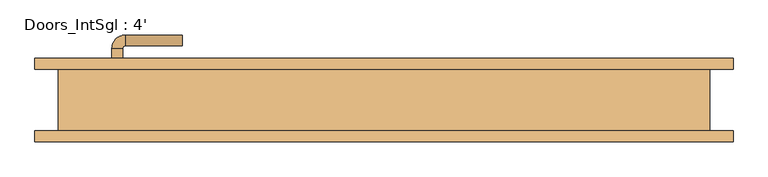
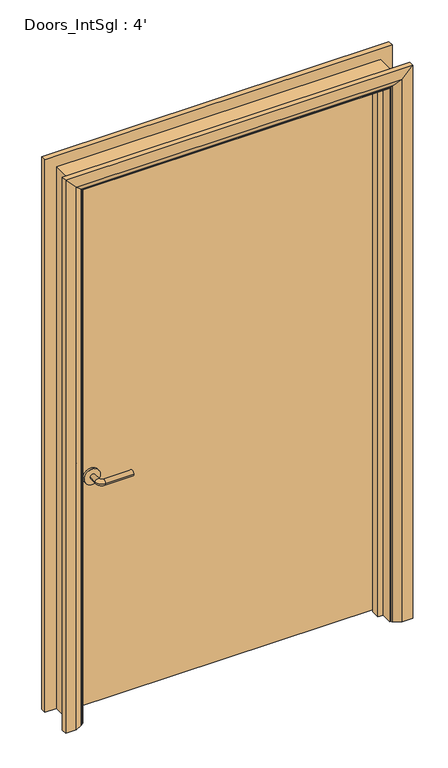
"""IFC4 building model written with IfcOpenShell, lengths in millimetres: door geometry, Doors_IntSgl : 4'."""

from ifc_helpers import new_model, si_unit, point, frame, frame_2d, origin, place, context, project, spatial, polyline, circle_curve, ellipse_curve, trimmed, segment, composite_curve, outline, extrude, faceted_brep, source, transform, mapped, element, save
from ifc_brep_helpers import plane_surface, cylinder_surface, revolved_surface, advanced_brep


def doors_intsgl_4_134d4d27(model_context):
    return source(origin(), model_context, "Body", "SolidModel", [
        advanced_brep(
        [(-502.6, 11.15, 900.0), (-482.6, 11.15, 900.0), (-482.6, -18.85, 900.0), (-502.6, -18.85, 900.0), (-477.6, -23.85, 900.0), (-477.6, -43.85, 900.0), (-372.6, -43.85, 900.0), (-372.6, -23.85, 900.0)],
        [
            (0, 1, circle_curve(frame((-492.6, 11.15, 900.0), z_axis=(0.0, 1.0, 0.0), x_axis=(1.0, 0.0, 0.0)), 10.0)),
            (1, 0, circle_curve(frame((-492.6, 11.15, 900.0), z_axis=(0.0, 1.0, 0.0), x_axis=(1.0, 0.0, 0.0)), 10.0)),
            (1, 2),
            (2, 3, circle_curve(frame((-492.6, -18.85, 900.0), z_axis=(0.0, 1.0, 0.0), x_axis=(1.0, 0.0, 0.0)), 10.0)),
            (3, 0),
            (3, 2, circle_curve(frame((-492.6, -18.85, 900.0), z_axis=(0.0, 1.0, 0.0), x_axis=(1.0, 0.0, 0.0)), 10.0)),
            (4, 5, circle_curve(frame((-477.6, -33.85, 900.0), z_axis=(-1.0, 0.0, 0.0), x_axis=(0.0, 1.0, 0.0)), 10.0)),
            (5, 3, circle_curve(frame((-477.6, -18.85, 900.0), z_axis=(0.0, 0.0, -1.0), x_axis=(-1.0, 0.0, 0.0)), 25.0)),
            (2, 4, circle_curve(frame((-477.6, -18.85, 900.0), z_axis=(0.0, 0.0, 1.0), x_axis=(-1.0, 0.0, 0.0)), 5.0)),
            (5, 4, circle_curve(frame((-477.6, -33.85, 900.0), z_axis=(-1.0, 0.0, 0.0), x_axis=(0.0, 1.0, 0.0)), 10.0)),
            (6, 7, circle_curve(frame((-372.6, -33.85, 900.0), z_axis=(1.0, 0.0, 0.0), x_axis=(0.0, 1.0, 0.0)), 10.0)),
            (7, 6, circle_curve(frame((-372.6, -33.85, 900.0), z_axis=(1.0, 0.0, 0.0), x_axis=(0.0, 1.0, 0.0)), 10.0)),
            (4, 7),
            (6, 5),
        ],
        [
            plane_surface(frame((-492.6, 11.15, 900.0), z_axis=(0.0, 1.0, 0.0), x_axis=(0.0, 0.0, 1.0))),
            cylinder_surface(frame((-492.6, 11.15, 900.0), z_axis=(0.0, 1.0, 0.0), x_axis=(1.0, 0.0, 0.0)), 10.0),
            revolved_surface(trimmed(ellipse_curve(frame((-492.6, -18.85, 900.0), z_axis=(0.0, -1.0, 0.0), x_axis=(1.0, 0.0, 0.0)), 10.0, 10.0), [point((-502.6, -18.85, 900.0))], [point((-482.6, -18.85, 900.0))], True, "CARTESIAN"), (-477.6, -18.85, 900.0), (0.0, 0.0, -1.0)),
            revolved_surface(trimmed(ellipse_curve(frame((-492.6, -18.85, 900.0), z_axis=(0.0, -1.0, 0.0), x_axis=(1.0, 0.0, 0.0)), 10.0, 10.0), [point((-482.6, -18.85, 900.0))], [point((-502.6, -18.85, 900.0))], True, "CARTESIAN"), (-477.6, -18.85, 900.0), (0.0, 0.0, -1.0)),
            plane_surface(frame((-372.6, -33.85, 900.0), z_axis=(1.0, 0.0, 0.0), x_axis=(0.0, 0.0, 1.0))),
            cylinder_surface(frame((-477.6, -33.85, 900.0), z_axis=(-1.0, 0.0, 0.0), x_axis=(0.0, 1.0, 0.0)), 10.0),
        ],
        [
            (0, [[1, 2]]),
            (1, [[3, 4, 5, -2]]),
            (1, [[-5, 6, -3, -1]]),
            (2, [[7, 8, -4, 9]]),
            (3, [[10, -9, -6, -8]]),
            (4, [[11, 12]]),
            (5, [[13, -11, 14, -7]]),
            (5, [[-14, -12, -13, -10]]),
        ],
    ),
        extrude(outline(composite_curve([segment(trimmed(circle_curve(frame_2d((900.0, -495.1)), 30.0), [point((900.0, -525.1))], [point((900.0, -465.1))], False, "CARTESIAN"), True, "CONTINUOUS"), segment(trimmed(circle_curve(frame_2d((900.0, -495.1)), 30.0), [point((900.0, -465.1))], [point((900.0, -525.1))], False, "CARTESIAN"), True, "CONTINUOUS")], self_intersect=False)), frame((0.0, 11.15, 0.0), z_axis=(0.0, 1.0, 0.0), x_axis=(0.0, 0.0, 1.0)), (0.0, 0.0, 1.0), 8.0),
        advanced_brep(
        [(-502.6, 65.15, 900.0), (-482.6, 65.15, 900.0), (-502.6, 95.15, 900.0), (-482.6, 95.15, 900.0), (-477.6, 100.15, 900.0), (-477.6, 120.15, 900.0), (-372.6, 120.15, 900.0), (-372.6, 100.15, 900.0)],
        [
            (0, 1, circle_curve(frame((-492.6, 65.15, 900.0), z_axis=(0.0, -1.0, 0.0), x_axis=(1.0, 0.0, 0.0)), 10.0)),
            (1, 0, circle_curve(frame((-492.6, 65.15, 900.0), z_axis=(0.0, -1.0, 0.0), x_axis=(1.0, 0.0, 0.0)), 10.0)),
            (0, 2),
            (2, 3, circle_curve(frame((-492.6, 95.15, 900.0), z_axis=(0.0, -1.0, 0.0), x_axis=(1.0, 0.0, 0.0)), 10.0)),
            (3, 1),
            (3, 2, circle_curve(frame((-492.6, 95.15, 900.0), z_axis=(0.0, -1.0, 0.0), x_axis=(1.0, 0.0, 0.0)), 10.0)),
            (4, 3, circle_curve(frame((-477.6, 95.15, 900.0), z_axis=(0.0, 0.0, 1.0), x_axis=(-1.0, 0.0, 0.0)), 5.0)),
            (2, 5, circle_curve(frame((-477.6, 95.15, 900.0), z_axis=(0.0, 0.0, -1.0), x_axis=(-1.0, 0.0, 0.0)), 25.0)),
            (5, 4, circle_curve(frame((-477.6, 110.15, 900.0), z_axis=(-1.0, 0.0, 0.0), x_axis=(0.0, -1.0, 0.0)), 10.0)),
            (4, 5, circle_curve(frame((-477.6, 110.15, 900.0), z_axis=(-1.0, 0.0, 0.0), x_axis=(0.0, -1.0, 0.0)), 10.0)),
            (6, 7, circle_curve(frame((-372.6, 110.15, 900.0), z_axis=(1.0, 0.0, 0.0), x_axis=(0.0, -1.0, 0.0)), 10.0)),
            (7, 6, circle_curve(frame((-372.6, 110.15, 900.0), z_axis=(1.0, 0.0, 0.0), x_axis=(0.0, -1.0, 0.0)), 10.0)),
            (5, 6),
            (7, 4),
        ],
        [
            plane_surface(frame((-492.6, 65.15, 900.0), z_axis=(0.0, -1.0, 0.0), x_axis=(0.0, 0.0, 1.0))),
            cylinder_surface(frame((-492.6, 65.15, 900.0), z_axis=(0.0, -1.0, 0.0), x_axis=(1.0, 0.0, 0.0)), 10.0),
            revolved_surface(trimmed(ellipse_curve(frame((-492.6, 95.15, 900.0), z_axis=(0.0, -1.0, 0.0), x_axis=(1.0, 0.0, 0.0)), 10.0, 10.0), [point((-502.6, 95.15, 900.0))], [point((-482.6, 95.15, 900.0))], True, "CARTESIAN"), (-477.6, 95.15, 900.0), (0.0, 0.0, -1.0)),
            revolved_surface(trimmed(ellipse_curve(frame((-492.6, 95.15, 900.0), z_axis=(0.0, -1.0, 0.0), x_axis=(1.0, 0.0, 0.0)), 10.0, 10.0), [point((-482.6, 95.15, 900.0))], [point((-502.6, 95.15, 900.0))], True, "CARTESIAN"), (-477.6, 95.15, 900.0), (0.0, 0.0, -1.0)),
            plane_surface(frame((-372.6, 110.15, 900.0), z_axis=(1.0, 0.0, 0.0), x_axis=(0.0, 0.0, 1.0))),
            cylinder_surface(frame((-477.6, 110.15, 900.0), z_axis=(-1.0, 0.0, 0.0), x_axis=(0.0, -1.0, 0.0)), 10.0),
        ],
        [
            (0, [[1, 2]]),
            (1, [[-1, 3, 4, 5]]),
            (1, [[-2, -5, 6, -3]]),
            (2, [[7, -4, 8, 9]]),
            (3, [[-8, -6, -7, 10]]),
            (4, [[11, 12]]),
            (5, [[-9, 13, -12, 14]]),
            (5, [[-10, -14, -11, -13]]),
        ],
    ),
        extrude(outline(composite_curve([segment(trimmed(circle_curve(frame_2d((900.0, -495.1)), 30.0), [point((900.0, -525.1))], [point((900.0, -465.1))], False, "CARTESIAN"), True, "CONTINUOUS"), segment(trimmed(circle_curve(frame_2d((900.0, -495.1)), 30.0), [point((900.0, -465.1))], [point((900.0, -525.1))], False, "CARTESIAN"), True, "CONTINUOUS")], self_intersect=False)), frame((0.0, 57.15, 0.0), z_axis=(0.0, 1.0, 0.0), x_axis=(0.0, 0.0, 1.0)), (0.0, 0.0, 1.0), 8.0),
        extrude(outline(polyline([(567.6, 19.15), (-567.6, 19.15), (-567.6, 57.15), (567.6, 57.15), (567.6, 19.15)])), frame((0.0, 0.0, 8.0), z_axis=(0.0, 0.0, 1.0), x_axis=(1.0, 0.0, 0.0)), (0.0, 0.0, 1.0), 2083.6),
        advanced_brep(
        [(644.6, 77.15, 0.0), (644.6, 57.15, 0.0), (574.6, 57.15, 0.0), (578.6, 63.15, 0.0), (604.6, 77.15, 0.0), (644.6, 77.15, 2168.6), (644.6, 57.15, 2168.6), (-644.6, 57.15, 2168.6), (-644.6, 57.15, 0.0), (-574.6, 57.15, 0.0), (-574.6, 57.15, 2098.6), (574.6, 57.15, 2098.6), (578.6, 63.15, 2102.6), (604.6, 77.15, 2128.6), (-604.6, 77.15, 2128.6), (-604.6, 77.15, 0.0), (-644.6, 77.15, 0.0), (-644.6, 77.15, 2168.6), (-578.6, 63.15, 0.0), (-578.6, 63.15, 2102.6)],
        [
            (0, 1),
            (1, 2),
            (2, 3, circle_curve(frame((582.6, 56.15, 0.0), z_axis=(0.0, 0.0, -1.0), x_axis=(1.0, 0.0, 0.0)), 8.0622577)),
            (3, 4),
            (4, 0),
            (0, 5),
            (5, 6),
            (6, 1),
            (6, 7),
            (7, 8),
            (8, 9),
            (9, 10),
            (10, 11),
            (11, 2),
            (11, 12, ellipse_curve(frame((582.6, 56.15, 2106.6), z_axis=(0.7071067811865475, 0.0, -0.7071067811865475), x_axis=(-0.7071067811865474, 0.0, -0.7071067811865476)), 11.4017543, 8.0622577)),
            (12, 3),
            (12, 13),
            (13, 4),
            (13, 14),
            (14, 15),
            (15, 16),
            (16, 17),
            (17, 5),
            (7, 17),
            (16, 8),
            (15, 18),
            (18, 9, circle_curve(frame((-582.6, 56.15, 0.0), z_axis=(0.0, 0.0, -1.0), x_axis=(-1.0, 0.0, 0.0)), 8.0622577)),
            (19, 10, ellipse_curve(frame((-582.6, 56.15, 2106.6), z_axis=(-0.7071067811865475, 0.0, -0.7071067811865475), x_axis=(-0.7071067811865474, 0.0, 0.7071067811865476)), 11.4017543, 8.0622577)),
            (18, 19),
            (14, 19),
            (19, 12),
        ],
        [
            plane_surface(frame((574.6, 57.15, 0.0), z_axis=(0.0, 0.0, -1.0), x_axis=(0.0, -1.0, 0.0))),
            plane_surface(frame((644.6, 77.15, 0.0), z_axis=(1.0, 0.0, 0.0), x_axis=(0.0, 0.0, 1.0))),
            plane_surface(frame((644.6, 57.15, 0.0), z_axis=(0.0, -1.0, 0.0), x_axis=(0.0, 0.0, 1.0))),
            cylinder_surface(frame((582.6, 56.15, 0.0), z_axis=(0.0, 0.0, -1.0), x_axis=(1.0, 0.0, 0.0)), 8.0622577),
            plane_surface(frame((578.6, 63.15, 0.0), z_axis=(-0.4740998230350126, 0.880471099922178, 0.0), x_axis=(0.0, 0.0, 1.0))),
            plane_surface(frame((604.6, 77.15, 0.0), z_axis=(0.0, 1.0, 0.0), x_axis=(0.0, 0.0, 1.0))),
            plane_surface(frame((-644.6, 77.15, 2168.6), z_axis=(-1.0, 0.0, 0.0), x_axis=(0.0, 0.0, -1.0))),
            plane_surface(frame((-574.6, 57.15, 0.0), z_axis=(0.0, 0.0, -1.0), x_axis=(0.0, -1.0, 0.0))),
            cylinder_surface(frame((-582.6, 56.15, 2098.6), z_axis=(0.0, 0.0, 1.0), x_axis=(-1.0, 0.0, 0.0)), 8.0622577),
            plane_surface(frame((-578.6, 63.15, 2102.6), z_axis=(0.47409982303501824, 0.8804710999221749, 0.0), x_axis=(0.0, 0.0, -1.0))),
            plane_surface(frame((644.6, 77.15, 2168.6), z_axis=(0.0, 0.0, 1.0), x_axis=(-1.0, 0.0, 0.0))),
            cylinder_surface(frame((574.6, 56.15, 2106.6), z_axis=(1.0, 0.0, 0.0), x_axis=(0.0, 0.0, 1.0)), 8.0622577),
            plane_surface(frame((578.6, 63.15, 2102.6), z_axis=(0.0, 0.8804710999221764, -0.4740998230350154), x_axis=(-1.0, 0.0, 0.0))),
        ],
        [
            (0, [[1, 2, 3, 4, 5]]),
            (1, [[-1, 6, 7, 8]]),
            (2, [[-2, -8, 9, 10, 11, 12, 13, 14]]),
            (3, [[-3, -14, 15, 16]]),
            (4, [[-4, -16, 17, 18]]),
            (5, [[-5, -18, 19, 20, 21, 22, 23, -6]]),
            (6, [[24, -22, 25, -10]]),
            (7, [[-21, 26, 27, -11, -25]]),
            (8, [[28, -12, -27, 29]]),
            (9, [[30, -29, -26, -20]]),
            (10, [[-7, -23, -24, -9]]),
            (11, [[-15, -13, -28, 31]]),
            (12, [[-17, -31, -30, -19]]),
        ],
    ),
        extrude(outline(polyline([(0.0, -569.6), (0.0, -550.6), (2074.6, -550.6), (2074.6, 550.6), (0.0, 550.6), (0.0, 569.6), (2093.6, 569.6), (2093.6, -569.6), (0.0, -569.6)])), frame((0.0, -14.85, 0.0), z_axis=(0.0, 1.0, 0.0), x_axis=(0.0, 0.0, 1.0)), (0.0, 0.0, 1.0), 32.0),
        advanced_brep(
        [(-644.6, -77.15, 0.0), (-644.6, -57.15, 0.0), (-574.6, -57.15, 0.0), (-578.6, -63.15, 0.0), (-604.6, -77.15, 0.0), (-644.6, -77.15, 2168.6), (-644.6, -57.15, 2168.6), (-574.6, -57.15, 2098.6), (-578.6, -63.15, 2102.6), (-604.6, -77.15, 2128.6), (644.6, -77.15, 0.0), (604.6, -77.15, 0.0), (578.6, -63.15, 0.0), (574.6, -57.15, 0.0), (644.6, -57.15, 0.0), (644.6, -77.15, 2168.6), (604.6, -77.15, 2128.6), (578.6, -63.15, 2102.6), (574.6, -57.15, 2098.6), (644.6, -57.15, 2168.6)],
        [
            (0, 1),
            (1, 2),
            (2, 3, circle_curve(frame((-582.6, -56.15, 0.0), z_axis=(0.0, 0.0, -1.0), x_axis=(-1.0, 0.0, 0.0)), 8.0622577)),
            (3, 4),
            (4, 0),
            (0, 5),
            (5, 6),
            (6, 1),
            (6, 7),
            (7, 2),
            (7, 8, ellipse_curve(frame((-582.6, -56.15, 2106.6), z_axis=(-0.7071067811865475, 0.0, -0.7071067811865475), x_axis=(0.7071067811865474, 0.0, -0.7071067811865476)), 11.4017543, 8.0622577)),
            (8, 3),
            (8, 9),
            (9, 4),
            (9, 5),
            (10, 11),
            (11, 12),
            (12, 13, circle_curve(frame((582.6, -56.15, 0.0), z_axis=(0.0, 0.0, -1.0), x_axis=(1.0, 0.0, 0.0)), 8.0622577)),
            (13, 14),
            (14, 10),
            (15, 16),
            (16, 11),
            (10, 15),
            (16, 17),
            (17, 12),
            (17, 18, ellipse_curve(frame((582.6, -56.15, 2106.6), z_axis=(0.7071067811865475, 0.0, -0.7071067811865475), x_axis=(0.7071067811865474, 0.0, 0.7071067811865476)), 11.4017543, 8.0622577)),
            (18, 13),
            (18, 19),
            (19, 14),
            (19, 15),
            (5, 15),
            (19, 6),
            (18, 7),
            (17, 8),
            (16, 9),
        ],
        [
            plane_surface(frame((-574.6, -129.9510989, 0.0), z_axis=(0.0, 0.0, -1.0), x_axis=(1.0, 0.0, 0.0))),
            plane_surface(frame((-644.6, -77.15, 0.0), z_axis=(-1.0, 0.0, 0.0), x_axis=(0.0, 0.0, 1.0))),
            plane_surface(frame((-644.6, -57.15, 0.0), z_axis=(0.0, 1.0, 0.0), x_axis=(0.0, 0.0, 1.0))),
            cylinder_surface(frame((-582.6, -56.15, 0.0), z_axis=(0.0, 0.0, -1.0), x_axis=(-1.0, 0.0, 0.0)), 8.0622577),
            plane_surface(frame((-578.6, -63.15, 0.0), z_axis=(0.4740998230350183, -0.8804710999221749, 0.0), x_axis=(0.0, 0.0, 1.0))),
            plane_surface(frame((-604.6, -77.15, 0.0), z_axis=(0.0, -1.0, 0.0), x_axis=(0.0, 0.0, 1.0))),
            plane_surface(frame((574.6, -129.9510989, 0.0), z_axis=(0.0, 0.0, -1.0), x_axis=(-1.0, 0.0, 0.0))),
            plane_surface(frame((604.6, -77.15, 2128.6), z_axis=(0.0, -1.0, 0.0), x_axis=(0.0, 0.0, -1.0))),
            plane_surface(frame((578.6, -63.15, 2102.6), z_axis=(-0.4740998230350183, -0.8804710999221749, 0.0), x_axis=(0.0, 0.0, -1.0))),
            cylinder_surface(frame((582.6, -56.15, 2098.6), z_axis=(0.0, 0.0, 1.0), x_axis=(1.0, 0.0, 0.0)), 8.0622577),
            plane_surface(frame((644.6, -57.15, 2168.6), z_axis=(0.0, 1.0, 0.0), x_axis=(0.0, 0.0, -1.0))),
            plane_surface(frame((644.6, -77.15, 2168.6), z_axis=(1.0, 0.0, 0.0), x_axis=(0.0, 0.0, -1.0))),
            plane_surface(frame((-644.6, -77.15, 2168.6), z_axis=(0.0, 0.0, 1.0), x_axis=(1.0, 0.0, 0.0))),
            plane_surface(frame((-644.6, -57.15, 2168.6), z_axis=(0.0, 1.0, 0.0), x_axis=(1.0, 0.0, 0.0))),
            cylinder_surface(frame((-574.6, -56.15, 2106.6), z_axis=(-1.0, 0.0, 0.0), x_axis=(0.0, 0.0, 1.0)), 8.0622577),
            plane_surface(frame((-578.6, -63.15, 2102.6), z_axis=(0.0, -0.8804710999221749, -0.4740998230350183), x_axis=(1.0, 0.0, 0.0))),
            plane_surface(frame((-604.6, -77.15, 2128.6), z_axis=(0.0, -1.0, 0.0), x_axis=(1.0, 0.0, 0.0))),
        ],
        [
            (0, [[1, 2, 3, 4, 5]]),
            (1, [[-1, 6, 7, 8]]),
            (2, [[-2, -8, 9, 10]]),
            (3, [[-3, -10, 11, 12]]),
            (4, [[-4, -12, 13, 14]]),
            (5, [[-5, -14, 15, -6]]),
            (6, [[16, 17, 18, 19, 20]]),
            (7, [[21, 22, -16, 23]]),
            (8, [[24, 25, -17, -22]]),
            (9, [[26, 27, -18, -25]]),
            (10, [[28, 29, -19, -27]]),
            (11, [[30, -23, -20, -29]]),
            (12, [[-7, 31, -30, 32]]),
            (13, [[-9, -32, -28, 33]]),
            (14, [[-11, -33, -26, 34]]),
            (15, [[-13, -34, -24, 35]]),
            (16, [[-15, -35, -21, -31]]),
        ],
    ),
        faceted_brep([(-569.6, 57.15, 0.0), (-569.6, -57.15, 0.0), (-601.6, -57.15, 0.0), (-601.6, 57.15, 0.0), (-569.6, 57.15, 2093.6), (-569.6, -57.15, 2093.6), (-601.6, -57.15, 2125.6), (-601.6, 57.15, 2125.6), (569.6, 57.15, 0.0), (601.6, 57.15, 0.0), (601.6, -57.15, 0.0), (569.6, -57.15, 0.0), (569.6, 57.15, 2093.6), (601.6, 57.15, 2125.6), (601.6, -57.15, 2125.6), (569.6, -57.15, 2093.6)], [[[0, 1, 2, 3]], [[1, 0, 4, 5]], [[2, 1, 5, 6]], [[3, 2, 6, 7]], [[0, 3, 7, 4]], [[8, 9, 10, 11]], [[12, 13, 9, 8]], [[13, 14, 10, 9]], [[14, 15, 11, 10]], [[15, 12, 8, 11]], [[5, 4, 12, 15]], [[6, 5, 15, 14]], [[7, 6, 14, 13]], [[4, 7, 13, 12]]]),
    ])


if __name__ == "__main__":
    model = new_model("IFC4")
    model_context = context("Model", 3, world=origin())
    ifc_project = project(units=[si_unit("LENGTHUNIT", "METRE", prefix="MILLI")], contexts=[model_context])
    site = spatial("IfcSite", under=ifc_project)
    building = spatial("IfcBuilding", under=site)
    placement = place(None, origin())
    doors_intsgl_4_shape = doors_intsgl_4_134d4d27(model_context)
    element("IfcDoor", 1, ObjectType="Doors_IntSgl : 4'", at=placement, inside=building, context=model_context, shape_type="MappedRepresentation", body=[
        mapped(doors_intsgl_4_shape, transform((0.0, 0.0, 0.0), x_axis=(1.0, 0.0, 0.0), y_axis=(0.0, 1.0, 0.0), z_axis=(0.0, 0.0, 1.0))),
    ])
    save(model, "model.ifc")

# Revit data of these elements
# Type "Doors_IntSgl : 4'"
#   Type Mark = "49"
#   Type Comments = "Internal Single"
#   Operation = "SingleSwingRight"
#   Manufacturer = "Revit"
#   Keynote = "L20"
#   Description = "Internal Single Door"
#   Analytic Construction = "Metal"
#   UnderCut = 0' - 0.31496"
#   Tolerance = 0' - 0.07874"
#   Thickness = 0' - 1.49606"
#   Thermal Resistance (R) = 0.270117 (m²·K)/W
#   Structural Tolerance = 0' - 0.31496"
#   StopDepth = 0' - 1.25984"
#   Stop Thickness = 0' - 0.74803"
#   Rough Width = 4' - 0"
#   Rough Height = 7' - 0"
#   Height to Top Lock Rail = 3' - 3.37008"
#   Heat Transfer Coefficient (U) = 3.7021 W/(m²·K)
#   Handle Z Distance = 2' - 11.43307"
#   Handle X Distance = 0' - 2.95276"
#   Frame Thickness = 0' - 1.25984"
#   Door Panel Width = 3' - 8.69291"
#   Door Panel Thickness = 0' - 1.49606"
#   Door Panel Offset = 0' - 0"
#   Height = 7' - 0"
#   Width = 4' - 0"
#   Door Panel Height = 6' - 10.0315"
#   Architrave Setback = 0' - 0.19685"
#   Vis - Ironmongery = yes
#   Material Ironmongery = Door - Handle
#   Material Frame = Door - Frame/Mullion (1)
#   Material Door = Door - Panel
#   Material Architrave = Door - Architrave
#   Visual Light Transmittance = 0
#   Solar Heat Gain Coefficient = 0
#   Function = (empty or 0)
#   Wall Closure = (empty or 0)
# Element 1 (IfcDoor, "Doors_IntSgl : 4'")
#   Materials on its faces: "Door - Architrave", "Door - Handle", "Door - Frame/Mullion (1)", "Door - Panel"
# Materials
#   "Door - Handle": colour RGB 0 0 0, transparency 0, Keynote = "P21", Cost = 0
#   "Door - Frame/Mullion (1)": class "Wood", colour RGB 212 179 113, transparency 0, Keynote = "L20", Cost = 0
#   "Door - Panel": class "Wood", colour RGB 210 159 95, transparency 0, Keynote = "L20", Cost = 0
#   "Door - Architrave": class "Wood", colour RGB 154 90 5, transparency 0, Keynote = "P20", Cost = 0
